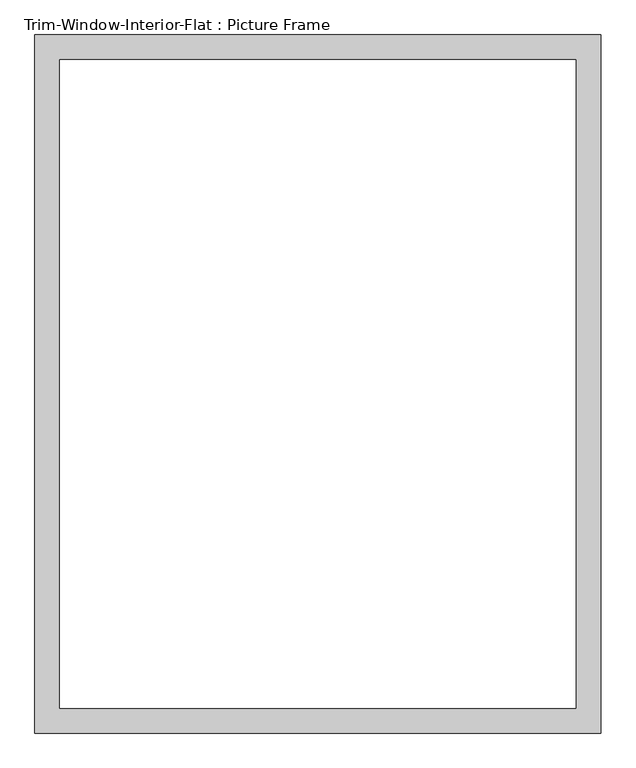
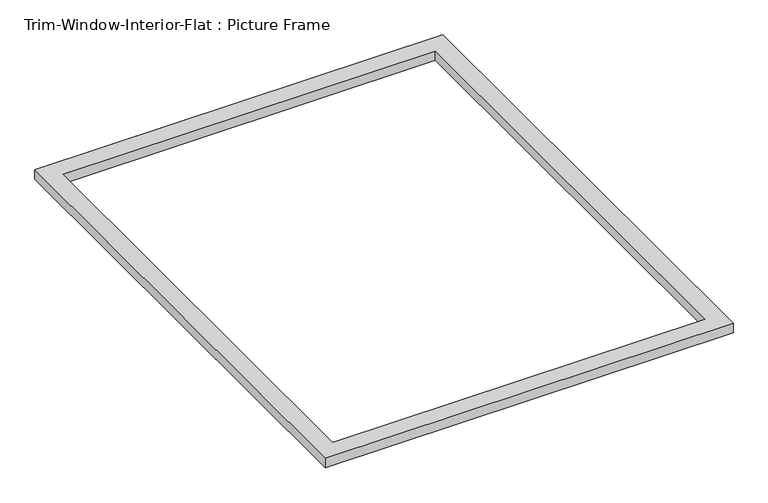
"""IFC4 building model written with IfcOpenShell, lengths in millimetres: proxy geometry, Trim-Window-Interior-Flat : Picture Frame."""

from ifc_helpers import new_model, si_unit, origin, origin_with_axes, place, context, project, spatial, polyline, outline, extrude, source, transform, mapped, element, save


def trim_window_interior_flat_picture_frame_3bb882cf(model_context):
    return source(origin(), model_context, "Body", "SweptSolid", [
        extrude(outline(polyline([(654.05, 44.45), (654.05, -1568.45), (-654.05, -1568.45), (-654.05, 44.45), (654.05, 44.45)]), holes=[polyline([(596.9, -12.7), (-596.9, -12.7), (-596.9, -1511.3), (596.9, -1511.3), (596.9, -12.7)])]), origin_with_axes(), (0.0, 0.0, 1.0), 31.75),
    ])


if __name__ == "__main__":
    model = new_model("IFC4")
    model_context = context("Model", 3, world=origin())
    ifc_project = project(units=[si_unit("LENGTHUNIT", "METRE", prefix="MILLI")], contexts=[model_context])
    site = spatial("IfcSite", under=ifc_project)
    building = spatial("IfcBuilding", under=site)
    placement = place(None, origin())
    trim_window_interior_flat_picture_frame_shape = trim_window_interior_flat_picture_frame_3bb882cf(model_context)
    element("IfcBuildingElementProxy", 1, Name="Trim-Window-Interior-Flat : Picture Frame", ObjectType="Trim-Window-Interior-Flat : Picture Frame", at=placement, inside=building, context=model_context, shape_type="MappedRepresentation", body=[
        mapped(trim_window_interior_flat_picture_frame_shape, transform((0.0, 0.0, 0.0), x_axis=(1.0, 0.0, 0.0), y_axis=(0.0, 1.0, 0.0), z_axis=(0.0, 0.0, 1.0))),
    ])
    save(model, "model.ifc")

# Revit data of these elements
# Type "Trim-Window-Interior-Flat : Picture Frame"
#   Trim Thickness_Picture Frame = 0' - 1 1/4"
#   Trim Width = 0' - 2 1/4"
#   Trim Thickness_with Sill = 0' - 0 3/4"
#   Sill Thickness = 0' - 1 1/4"
#   Opening Width [instance default] = 2' - 0"
#   Opening Height [instance default] = 3' - 0"
#   Default Elevation = 4' - 0"
#   Sill = no
#   Picture Frame = yes
#   Trim Material [instance default] = none
# Element 1 (IfcBuildingElementProxy, "Trim-Window-Interior-Flat : Picture Frame")
#   Opening Width = 4' - 0"
#   Opening Height = 5' - 0"
#   Trim Material = Wood - Stained
#   Materials on its faces: "Wood - Stained"
# Materials
#   "Wood - Stained": class "Wood", colour RGB 173 132 96, transparency 0, Cost = 0
